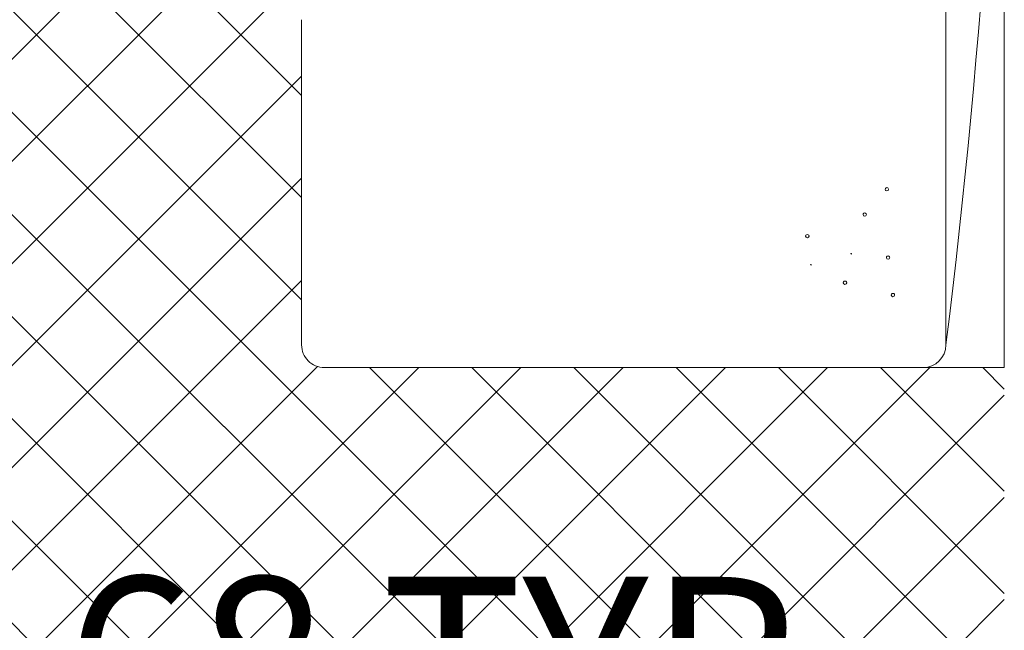
# Model space of a CAD drawing. Units: inches. Extents: x -466983 to 1020, y 324 to 318697.
# Tile 88 of 97: x 776 to 810, y 879 to 900. Entities that reach past the tile are written whole.
import ezdxf

# ---------------------------------------------------------------- set-up
doc = ezdxf.new("R2010")
doc.units = ezdxf.units.IN
doc.header["$MEASUREMENT"] = 0
for name, color, linetype, lineweight in [('A-ANNO-DIMS', 2, 'Continuous', 18), ('A-FLOR-PATT', 252, 'Continuous', 13), ('A-FURN', 8, 'Continuous', 18)]:
    doc.layers.add(name, color=color, linetype=linetype, lineweight=lineweight)
doc.styles.get("Standard").update_dxf_attribs({"font": 'arial.ttf'})
doc.dimstyles.get("Standard").update_dxf_attribs({"dimtxt": 6, "dimasz": 4, "dimexe": 3, "dimexo": 3, "dimgap": 0.09, "dimtad": 0, "dimtih": 1, "dimtoh": 1, "dimdec": 1, "dimzin": 0, "dimdsep": 46, "dimlunit": 3, "dimtxsty": 'Standard', "dimcen": 0.09, "dimadec": 0, "dimazin": 0, "dimtfac": 1, "dimtdec": 1, "dimtofl": 0, "dimtmove": 0, "dimatfit": 3, "dimfxl": 1, "dimtolj": 1, "dimtzin": 0, "dimarcsym": 0})

# ---------------------------------------------------------------- blocks, each defined once
blk = doc.blocks.new('L Shaped Sofa')
at = {"ltscale": 2}
for p, q in [((2356.696, 767.567), (2377.232, 767.567)), ((2355.263, 760.482), (2355.263, 766.134)), ((2355.263, 760.482), (2355.263, 736.259)), ((2355.263, 728.35), (2355.263, 736.259)), ((2355.263, 723.229), (2355.263, 728.35)), ((2356.696, 726.917), (2377.232, 726.917)), ((2393.28, 726.917), (2377.232, 726.917)), ((2355.263, 723.229), (2377.232, 723.229)), ((2475.263, 723.229), (2377.232, 723.229))]:
    blk.add_line(p, q, dxfattribs=at)
for centre, radius, start, end in [((2356.696, 766.134), 1.433, 90, 180), ((2363.564, 735.657), 0.106, 90, 270), ((2363.564, 735.657), 0.106, 270, 90), ((2361.755, 735.431), 0.0177, 90, 270), ((2361.755, 735.431), 0.0177, 270, 90), ((2360.624, 733.281), 0.106, 90, 270), ((2360.624, 733.281), 0.106, 270, 90), ((2362.453, 732.887), 0.0177, 90, 270), ((2362.453, 732.887), 0.0177, 270, 90), ((2364.92, 732.036), 0.106, 90, 270), ((2364.92, 732.036), 0.106, 270, 90), ((2362.207, 730.566), 0.106, 90, 270), ((2362.207, 730.566), 0.106, 270, 90), ((2366.526, 730.64), 0.106, 90, 270), ((2366.526, 730.64), 0.106, 270, 90), ((2359.842, 730.258), 0.106, 90, 270), ((2359.842, 730.258), 0.106, 270, 90), ((2356.696, 728.35), 1.433, 180, 270), ((2416.36, 1205.029), 481.82, 262.88673, 276.63201)]:
    blk.add_arc(centre, radius, start, end, dxfattribs=at)
blk = doc.blocks.new('*D71')
at = {"layer": 'A-ANNO-DIMS', "color": 0, "lineweight": -2, "transparency": 16777216}
for p, q in [((742.215, 885.152), (742.215, 874.91)), ((810.492, 885.152), (810.492, 874.91)), ((738.215, 877.91), (734.215, 877.91)), ((814.492, 877.91), (818.492, 877.91))]:
    blk.add_line(p, q, dxfattribs=at)
at = {"layer": 'A-ANNO-DIMS', "color": 0, "transparency": 16777216}
for points in [[(738.215, 878.577), (738.215, 877.244), (742.215, 877.91)], [(814.492, 878.577), (814.492, 877.244), (810.492, 877.91)]]:
    blk.add_solid(points, dxfattribs=at)
at = {"layer": 'Defpoints', "color": 0, "transparency": 16777216}
for p in [(742.215, 888.152), (810.492, 888.152), (742.215, 877.91)]:
    blk.add_point(p, dxfattribs=at)
at = {"layer": 'A-ANNO-DIMS', "color": 0, "transparency": 16777216, "insert": (776.354, 877.91), "char_height": 6, "attachment_point": 5}
blk.add_mtext('\\A1;L-SOFA 68 TYP.', dxfattribs=at)

msp = doc.modelspace()

# ---------------------------------------------------------------- hatches: boundary and pattern name
at = {"layer": 'A-FLOR-PATT', "transparency": 33554572}
h = msp.add_hatch(dxfattribs=at)
h.set_pattern_fill('ANSI37', color=256, scale=30)
h.set_pattern_definition([(45, (-1212.4137, -290.035), (-2.6516504, 2.6516504), []), (135, (-1212.4137, -290.035), (-2.6516504, -2.6516504), [])])
h.paths.add_polyline_path([(901.806, 1075.938), (900.614, 1075.938), (900.614, 1065.386), (899.391, 1065.386), (898.091, 1065.386), (892.836, 1058.71, -0.258377), (892.188, 1058.351), (879.985, 1058.351, -0.20177), (879.438, 1058.581), (874.081, 1065.386), (872.781, 1065.386), (871.558, 1065.386), (871.558, 1075.938), (813.806, 1075.938), (813.806, 1044.792), (832.395, 1044.792, -0.394795), (848.66, 1028.536), (848.66, 1009.938), (901.806, 1009.938), (901.806, 1015.938), (901.306, 1015.938), (871.306, 1015.938), (871.306, 1017.25), (871.334, 1017.25, -0.401453), (901.306, 1045.938), (901.806, 1045.938)])
edge = h.paths.add_edge_path(flags=16)
edge.add_line((847.773, 1068.949), (847.773, 1073.709))
edge.add_arc((849.227, 1073.709), 1.454, 90, 180, ccw=False)
edge.add_line((849.227, 1075.163), (864.492, 1075.163))
edge.add_arc((864.492, 1073.709), 1.454, 0, 90, ccw=False)
edge.add_line((865.946, 1073.709), (865.946, 1069.004))
edge.add_arc((832.645, 1068.976), 33.301, -20.6123, 0.0472, ccw=False)
edge.add_ellipse((856.859, 1058.48), major_axis=(0, 10.213), ratio=0.685919, start_angle=100.0088, end_angle=259.9912, ccw=False)
edge.add_arc((881.074, 1068.976), 33.301, 180.0472, 200.6123, ccw=False)
h.paths.add_polyline_path([(853.146, 1066.482), (853.146, 1066.453), (853.146, 1066.453, 0.433107), (852.917, 1066.685), (852.917, 1066.453), (853.146, 1066.453), (853.146, 1066.482), (853.088, 1066.612, 0.697939), (852.7, 1066.453), (852.7, 1066.453), (852.7, 1066.482), (852.917, 1067.001), (852.917, 1066.685, -0.396254)], flags=0)
h.paths.add_polyline_path([(861.019, 1066.482), (861.019, 1066.453), (861.019, 1066.453, 0.416404), (860.802, 1066.685), (860.802, 1066.453), (861.019, 1066.453), (861.019, 1066.482), (860.967, 1066.605, 0.713344), (860.573, 1066.453), (860.573, 1066.453), (860.573, 1066.482), (860.802, 1067.001), (860.802, 1066.685, -0.379973)], flags=0)
edge = h.paths.add_edge_path(flags=0)
edge.add_spline(control_points=[(861.13, 1065.785), (861.466, 1065.248), (861.613, 1065.016), (861.983, 1064.374), (862.192, 1063.944), (862.561, 1063.039), (862.721, 1062.563), (862.987, 1061.578), (863.092, 1061.069), (863.245, 1060.031), (863.293, 1059.503), (863.329, 1058.441), (863.318, 1057.908), (863.237, 1056.852), (863.166, 1056.329), (862.97, 1055.308), (862.843, 1054.81), (862.537, 1053.852), (862.357, 1053.393), (861.951, 1052.525), (861.725, 1052.117), (861.233, 1051.362), (860.967, 1051.016), (860.405, 1050.395), (860.108, 1050.12), (859.494, 1049.646), (859.176, 1049.448), (858.528, 1049.13), (858.197, 1049.011), (857.531, 1048.852), (857.196, 1048.812), (856.525, 1048.812), (856.189, 1048.852), (855.524, 1049.01), (855.193, 1049.129), (854.545, 1049.447), (854.227, 1049.645), (853.612, 1050.118), (853.316, 1050.393), (852.753, 1051.014), (852.487, 1051.36), (851.995, 1052.114), (851.769, 1052.523), (851.363, 1053.39), (851.183, 1053.85), (850.877, 1054.807), (850.75, 1055.305), (850.553, 1056.326), (850.483, 1056.849), (850.401, 1057.905), (850.39, 1058.438), (850.426, 1059.5), (850.473, 1060.028), (850.626, 1061.066), (850.732, 1061.575), (850.997, 1062.561), (851.157, 1063.036), (851.525, 1063.942), (851.734, 1064.371), (852.106, 1065.016), (852.254, 1065.25), (852.608, 1065.733)], knot_values=[3.915332, 3.915332, 3.915332, 3.915332, 4.013468, 4.013468, 4.175532, 4.175532, 4.337596, 4.337596, 4.49966, 4.49966, 4.661724, 4.661724, 4.823788, 4.823788, 4.985852, 4.985852, 5.147916, 5.147916, 5.30998, 5.30998, 5.472044, 5.472044, 5.634109, 5.634109, 5.796173, 5.796173, 5.958237, 5.958237, 6.120301, 6.120301, 6.282365, 6.282365, 6.444429, 6.444429, 6.606493, 6.606493, 6.768557, 6.768557, 6.930621, 6.930621, 7.092685, 7.092685, 7.254749, 7.254749, 7.416813, 7.416813, 7.578878, 7.578878, 7.740942, 7.740942, 7.903006, 7.903006, 8.06507, 8.06507, 8.227134, 8.227134, 8.389198, 8.389198, 8.551262, 8.551262, 8.65037, 8.65037, 8.65037, 8.65037], degree=3, periodic=0)
edge.add_line((852.642, 1065.785), (861.13, 1065.785))
edge = h.paths.add_edge_path(flags=0)
edge.add_ellipse((856.85, 1057.743), major_axis=(0, 7.792), ratio=0.687861, start_angle=0, end_angle=360)
h.paths.add_polyline_path([(848.863, 1069.389), (848.863, 1073.96, -0.414214), (849.954, 1075.051), (863.765, 1075.051, -0.414214), (864.856, 1073.96), (864.856, 1069.389, -0.388936), (864.524, 1069.027, -0.043561), (849.195, 1069.027, -0.388936)], flags=0)
h.paths.add_polyline_path([(853.101, 1068.112, -1), (852.677, 1068.112, -1)], flags=0)
edge = h.paths.add_edge_path(flags=0)
edge.add_ellipse((856.859, 1057.338), major_axis=(0, 2.207), ratio=0.657164, start_angle=0, end_angle=360)
h.paths.add_polyline_path([(861.041, 1068.112, -1), (860.618, 1068.112, -1)], flags=0)
edge = h.paths.add_edge_path()
edge.add_line((573.954, 1057.341), (573.954, 1075.938))
edge.add_line((573.954, 1075.938), (558.731, 1075.938))
edge.add_line((558.731, 1075.938), (558.731, 1065.386))
edge.add_line((558.731, 1065.386), (557.507, 1065.386))
edge.add_line((557.507, 1065.386), (556.207, 1065.386))
edge.add_line((556.207, 1065.386), (550.952, 1058.71))
edge.add_arc((550.304, 1059.116), 0.765, 270, 327.9483, ccw=False)
edge.add_line((550.304, 1058.351), (538.101, 1058.351))
edge.add_arc((538.101, 1059.116), 0.765, 224.3704, 270, ccw=False)
edge.add_line((537.555, 1058.581), (532.198, 1065.386))
edge.add_line((532.198, 1065.386), (530.898, 1065.386))
edge.add_line((530.898, 1065.386), (529.674, 1065.386))
edge.add_line((529.674, 1065.386), (529.674, 1075.938))
edge.add_line((529.674, 1075.938), (520.806, 1075.938))
edge.add_line((520.806, 1075.938), (520.806, 1045.938))
edge.add_line((520.806, 1045.938), (521.306, 1045.938))
edge.add_arc((521.306, 1015.938), 30, 2.5075, 90, ccw=False)
edge.add_line((551.277, 1017.25), (551.306, 1017.25))
edge.add_line((551.306, 1017.25), (551.306, 1015.938))
edge.add_line((551.306, 1015.938), (520.806, 1015.938))
edge.add_line((520.806, 1015.938), (520.806, 1009.938))
edge.add_line((520.806, 1009.938), (559.191, 1010.402))
edge.add_arc((559.191, 1011.856), 1.454, 180, 270, ccw=False)
edge.add_line((557.737, 1011.856), (557.737, 1016.561))
edge.add_arc((591.039, 1016.589), 33.301, 159.3877, 180.0472, ccw=False)
edge.add_ellipse((566.824, 1027.085), major_axis=(0, 10.213), ratio=0.685919, start_angle=280.0088, end_angle=439.9912, ccw=False)
edge.add_arc((542.609, 1016.589), 33.301, 0.0472, 20.6123, ccw=False)
edge.add_line((575.91, 1016.616), (575.91, 1011.856))
edge.add_arc((574.456, 1011.856), 1.454, -90, 0, ccw=False)
edge.add_line((574.456, 1010.402), (608.806, 1009.938))
edge.add_line((608.806, 1009.938), (608.806, 1041.086))
edge.add_line((608.806, 1041.086), (590.218, 1041.086))
edge.add_arc((590.775, 1057.907), 16.831, 181.9277, 268.1032, ccw=False)
edge = h.paths.add_edge_path()
edge.add_ellipse((494.244, 583.62), major_axis=(0, 10.213), ratio=0.685919, start_angle=280.0088, end_angle=439.9912, ccw=False)
edge.add_arc((470.03, 573.124), 33.301, 0.0472, 20.6123, ccw=False)
edge.add_line((503.331, 573.152), (503.331, 568.392))
edge.add_arc((501.877, 568.392), 1.454, -90, 0, ccw=False)
edge.add_line((501.877, 566.938), (539.806, 566.938))
edge.add_line((539.806, 566.938), (539.806, 572.938))
edge.add_line((539.806, 572.938), (539.306, 572.938))
edge.add_line((539.306, 572.938), (509.306, 572.938))
edge.add_line((509.306, 572.938), (509.306, 574.25))
edge.add_line((509.306, 574.25), (509.334, 574.25))
edge.add_arc((539.306, 572.938), 30, 90, 177.4925, ccw=False)
edge.add_line((539.306, 602.938), (539.806, 602.938))
edge.add_line((539.806, 602.938), (539.806, 626.938))
edge.add_line((539.806, 626.938), (531.772, 626.938))
edge.add_line((531.772, 626.938), (531.772, 616.386))
edge.add_line((531.772, 616.386), (530.548, 616.386))
edge.add_line((530.548, 616.386), (529.249, 616.386))
edge.add_line((529.249, 616.386), (523.711, 609.351))
edge.add_line((523.711, 609.351), (510.777, 609.351))
edge.add_line((510.777, 609.351), (505.239, 616.386))
edge.add_line((505.239, 616.386), (503.939, 616.386))
edge.add_line((503.939, 616.386), (502.715, 616.386))
edge.add_line((502.715, 616.386), (502.715, 626.938))
edge.add_line((502.715, 626.938), (481.698, 626.938))
edge.add_line((481.698, 626.938), (481.698, 610.995))
edge.add_arc((467.27, 611.473), 14.436, 271.9277, 358.1032, ccw=False)
edge.add_line((467.756, 597.045), (451.806, 597.045))
edge.add_line((451.806, 597.045), (451.806, 584.404))
edge.add_line((451.806, 584.404), (451.806, 566.938))
edge.add_line((451.806, 566.938), (486.612, 566.938))
edge.add_arc((486.612, 568.392), 1.454, 180, 270, ccw=False)
edge.add_line((485.158, 568.392), (485.158, 573.097))
edge.add_arc((518.459, 573.124), 33.301, 159.3877, 180.0472, ccw=False)
h.paths.add_polyline_path([(836.261, 1020.733), (879.89, 1020.733), (879.89, 1039.39), (836.261, 1039.39)], flags=25)
h.paths.add_polyline_path([(549.985, 1036.749), (593.614, 1036.749), (593.614, 1055.407), (549.985, 1055.407)], flags=24)
h.paths.add_polyline_path([(475.123, 595.596), (518.752, 595.596), (518.752, 614.253), (475.123, 614.253)], flags=24)
h = msp.add_hatch(dxfattribs=at)
h.set_pattern_fill('ANSI37', color=256, scale=20)
h.set_pattern_definition([(45, (-1212.4137, -290.035), (-1.767767, 1.767767), []), (135, (-1212.4137, -290.035), (-1.767767, -1.767767), [])])
h.paths.add_polyline_path([(809.806, 870.938), (809.806, 888.152), (806.998, 888.152), (802.662, 888.152), (789.383, 888.152), (786.285, 888.152, -0.414214), (785.499, 888.937), (785.499, 900.196), (785.499, 908.47, -0.414214), (786.808, 909.779, -0.414214), (785.499, 911.088), (785.499, 929.101, -0.414214), (786.808, 930.411, -0.414214), (785.499, 931.72), (785.499, 931.904, -0.414214), (784.19, 930.595), (766.722, 930.595, -0.412359), (765.413, 931.896, -0.413741), (764.115, 930.578), (744.578, 930.422, -0.416556), (743.786, 931.207), (743.786, 933.515), (742.215, 933.515), (742.215, 952.024, -0.001344), (743.786, 952.2), (743.786, 953.938), (678.592, 953.938), (678.592, 951.131), (678.592, 946.794), (678.592, 933.515), (678.592, 930.417, -0.414214), (677.806, 929.631), (666.548, 929.631), (658.274, 929.631, -0.414214), (656.965, 930.94, -0.414214), (655.656, 929.631), (637.642, 929.631, -0.414214), (636.333, 930.94, -0.414214), (635.024, 929.631), (634.839, 929.631, -0.414214), (636.149, 928.322), (636.149, 910.854, -0.412359), (634.848, 909.545, -0.413741), (636.165, 908.247), (636.321, 888.71, -0.416556), (635.536, 887.918), (633.228, 887.918), (633.228, 886.347), (614.719, 886.347, -0.001344), (614.544, 887.918), (612.806, 887.918), (612.806, 834.938), (612.806, 752.938), (612.806, 748.938), (612.806, 697.938), (654.806, 697.938), (654.806, 701.938), (715.806, 701.938), (715.806, 737.435), (774.292, 737.435), (774.292, 795.938), (809.806, 795.938)])
h.paths.add_polyline_path([(679.276, 849.576, 0.102523), (682.148, 849.261, -0.080461), (694.543, 849.773, -0.283899), (694.482, 849.008, 0.136605), (694.407, 848.81, -0.030441), (694.543, 846.893), (694.543, 842.62), (694.543, 838.347, -0.028219), (694.425, 836.568), (694.425, 836.568, 0.196187), (694.446, 836.271, -0.302897), (694.543, 835.467, -0.080461), (682.148, 835.979, 0.102523), (679.276, 835.664, -0.58611), (678.646, 836.017), (678.646, 849.223, -0.58611)], flags=16)
h.paths.add_polyline_path([(679.517, 848.651, 0.699597), (679.476, 848.634, 1.20716), (679.194, 848.742, 0.010621)], flags=0)
h.paths.add_polyline_path([(679.492, 836.561, -0.013798), (679.918, 836.659, -0.071703), (682.853, 837.143, -0.165743), (682.166, 839.101), (682.166, 842.609), (682.166, 846.06, -0.240616), (683.473, 848.677, -0.068263), (693.929, 849.008), (693.788, 848.708), (693.788, 849.023, 0.067332), (683.473, 848.677, 0.240616), (682.166, 846.06), (682.166, 842.609), (682.166, 839.101, 0.23459), (683.461, 836.551, 0.068093), (693.788, 836.195), (693.788, 836.51), (693.93, 836.21, -0.077215), (682.242, 836.782, 0.086627), (679.528, 836.57, -0.628402), (679.503, 836.573), (679.503, 836.607, 0.910458)], flags=0)
h.paths.add_polyline_path([(679.476, 848.636), (679.207, 848.647), (679.207, 836.572, 0.913566), (679.365, 836.586), (679.476, 836.582)], flags=0)
h.paths.add_polyline_path([(679.276, 829.86, 0.102523), (682.148, 829.546, -0.080461), (694.543, 830.057, -0.283899), (694.482, 829.293, 0.136605), (694.407, 829.095, -0.030441), (694.543, 827.178), (694.543, 822.904), (694.543, 818.631, -0.028219), (694.425, 816.853), (694.425, 816.853, 0.196187), (694.446, 816.556, -0.302897), (694.543, 815.752, -0.080461), (682.148, 816.263, 0.102523), (679.276, 815.949, -0.58611), (678.646, 816.302), (678.646, 829.507, -0.58611)], flags=16)
h.paths.add_polyline_path([(679.517, 828.936, 0.699597), (679.476, 828.919, 1.20716), (679.194, 829.027, 0.010621)], flags=0)
h.paths.add_polyline_path([(679.492, 816.846, -0.013798), (679.918, 816.944, -0.071703), (682.853, 817.428, -0.165743), (682.166, 819.385), (682.166, 822.894), (682.166, 826.345, -0.240616), (683.473, 828.961, -0.068263), (693.929, 829.293), (693.788, 828.993), (693.788, 829.308, 0.067332), (683.473, 828.961, 0.240616), (682.166, 826.345), (682.166, 822.894), (682.166, 819.385, 0.23459), (683.461, 816.836, 0.068093), (693.788, 816.48), (693.788, 816.795), (693.93, 816.495, -0.077215), (682.242, 817.066, 0.086627), (679.528, 816.855, -0.628402), (679.503, 816.858), (679.503, 816.892, 0.910458)], flags=0)
h.paths.add_polyline_path([(679.476, 828.921), (679.207, 828.932), (679.207, 816.857, 0.913566), (679.365, 816.871), (679.476, 816.867)], flags=0)
h.paths.add_polyline_path([(679.276, 810.145, 0.102523), (682.148, 809.83, -0.080461), (694.543, 810.342, -0.3023), (694.447, 809.539, 0.10023), (694.406, 809.388, -0.03057), (694.543, 807.462), (694.543, 803.189), (694.543, 798.916, -0.03057), (694.406, 796.991, 0.10023), (694.447, 796.839, -0.3023), (694.543, 796.036, -0.080461), (682.148, 796.548, 0.102523), (679.276, 796.233, -0.58611), (678.646, 796.586), (678.646, 809.792, -0.58611)], flags=16)
h.paths.add_polyline_path([(679.517, 809.242, 0.699597), (679.476, 809.224, 1.20716), (679.194, 809.332, 0.010621)], flags=0)
h.paths.add_polyline_path([(679.492, 797.151, -0.013798), (679.918, 797.25, -0.071703), (682.853, 797.734, -0.165743), (682.166, 799.691), (682.166, 803.2), (682.166, 806.65, -0.239349), (683.461, 809.258, -0.072465), (694.447, 809.541, 0.197932), (694.425, 809.241), (693.788, 809.299), (693.788, 809.614, 0.068093), (683.461, 809.258, 0.239349), (682.166, 806.65), (682.166, 803.2), (682.166, 799.691, 0.235854), (683.473, 797.132, 0.067332), (693.788, 796.786), (693.788, 797.101), (694.425, 797.159, 0.197932), (694.447, 796.859, -0.080419), (682.156, 797.379, 0.083867), (679.528, 797.16, -0.628402), (679.503, 797.164), (679.503, 797.197, 0.910458)], flags=0)
h.paths.add_polyline_path([(679.207, 809.237), (679.207, 797.162, 0.913566), (679.365, 797.176), (679.476, 797.173), (679.476, 809.227)], flags=0)
h.paths.add_polyline_path([(695.364, 853.299), (728.223, 853.299), (728.223, 771.152), (695.364, 771.152)], flags=16)
h.paths.add_polyline_path([(696.021, 852.642), (727.566, 852.642), (727.566, 771.809), (696.021, 771.809)], flags=0)
h.paths.add_polyline_path([(679.276, 788.787, 0.102523), (682.148, 788.472, -0.080461), (694.543, 788.984, -0.3023), (694.447, 788.181, 0.10023), (694.406, 788.03, -0.03057), (694.543, 786.104), (694.543, 781.831), (694.543, 777.558, -0.03057), (694.406, 775.632, 0.10023), (694.447, 775.481, -0.3023), (694.543, 774.678, -0.080461), (682.148, 775.19, 0.102523), (679.276, 774.875, -0.58611), (678.646, 775.228), (678.646, 788.434, -0.58611)], flags=16)
h.paths.add_polyline_path([(679.517, 787.883, 0.699597), (679.476, 787.866, 1.20716), (679.194, 787.974, 0.010621)], flags=0)
h.paths.add_polyline_path([(679.492, 775.793, -0.013798), (679.918, 775.891, -0.071703), (682.853, 776.375, -0.165743), (682.166, 778.333), (682.166, 781.841), (682.166, 785.292, -0.239349), (683.461, 787.899, -0.072465), (694.447, 788.182, 0.197932), (694.425, 787.882), (693.788, 787.94), (693.788, 788.255, 0.068093), (683.461, 787.899, 0.239349), (682.166, 785.292), (682.166, 781.841), (682.166, 778.333, 0.235854), (683.473, 775.774, 0.067332), (693.788, 775.428), (693.788, 775.742), (694.425, 775.8, 0.197932), (694.447, 775.5, -0.080419), (682.156, 776.021, 0.083867), (679.528, 775.802, -0.628402), (679.503, 775.805), (679.503, 775.839, 0.910458)], flags=0)
h.paths.add_polyline_path([(679.207, 787.879), (679.207, 775.804, 0.913566), (679.365, 775.818), (679.476, 775.814), (679.476, 787.868)], flags=0)
h.paths.add_polyline_path([(704.641, 854.12, -0.080461), (705.153, 866.516, 0.102523), (704.838, 869.387, -0.58611), (705.191, 870.017), (718.397, 870.017, -0.58611), (718.75, 869.387, 0.102523), (718.435, 866.516, -0.080461), (718.946, 854.12, -0.3023), (718.144, 854.217, 0.10023), (717.992, 854.257, -0.03057), (716.067, 854.12), (711.794, 854.12), (707.521, 854.12, -0.03057), (705.595, 854.257, 0.10023), (705.444, 854.217, -0.3023)], flags=16)
h.paths.add_polyline_path([(717.846, 869.146, 0.699597), (717.829, 869.187, 1.20716), (717.937, 869.47, 0.010621)], flags=0)
h.paths.add_polyline_path([(705.463, 854.216, -0.080419), (705.984, 866.507, 0.083867), (705.765, 869.135, -0.628402), (705.768, 869.16), (705.802, 869.16, 0.910458), (705.756, 869.171, -0.013798), (705.854, 868.745, -0.071703), (706.338, 865.81, -0.165743), (708.295, 866.497), (711.804, 866.497), (715.255, 866.497, -0.239349), (717.862, 865.202, -0.072465), (718.145, 854.216, 0.197932), (717.845, 854.238), (717.903, 854.876), (718.218, 854.876, 0.068093), (717.862, 865.202, 0.239349), (715.255, 866.497), (711.804, 866.497), (708.295, 866.497, 0.235854), (705.737, 865.19, 0.067332), (705.391, 854.876), (705.705, 854.876), (705.763, 854.238, 0.197932)], flags=16)
h.paths.add_polyline_path([(705.766, 869.456, 0.913566), (705.781, 869.299), (705.777, 869.187), (717.831, 869.187), (717.842, 869.456)], flags=0)
h.paths.add_polyline_path([(729.045, 842.62), (729.045, 846.893, -0.03057), (729.182, 848.818, 0.10023), (729.141, 848.97, -0.3023), (729.045, 849.773, -0.080461), (741.44, 849.261, 0.102523), (744.311, 849.576, -0.58611), (744.942, 849.223), (744.942, 836.017, -0.58611), (744.311, 835.664, 0.102523), (741.44, 835.979, -0.080461), (729.045, 835.467, -0.3023), (729.141, 836.27, 0.10023), (729.182, 836.421, -0.03057), (729.045, 838.347)], flags=16)
h.paths.add_polyline_path([(744.111, 836.585, 1.20716), (744.394, 836.477, 0.010621), (744.07, 836.567, 0.699597)], flags=0)
h.paths.add_polyline_path([(729.141, 836.268, 0.197932), (729.162, 836.568), (729.8, 836.51), (729.8, 836.195, 0.068093), (740.126, 836.551, 0.239349), (741.421, 839.159), (741.421, 842.609), (741.421, 846.118, 0.235854), (740.114, 848.677, 0.067332), (729.8, 849.023), (729.8, 848.708), (729.162, 848.65, 0.197932), (729.141, 848.95, -0.080419), (741.432, 848.43, 0.083867), (744.059, 848.649, -0.628402), (744.085, 848.645), (744.085, 848.612, 0.910458), (744.095, 848.658, -0.013798), (743.67, 848.559, -0.071703), (740.734, 848.075, -0.165743), (741.421, 846.118), (741.421, 842.609), (741.421, 839.159, -0.239349), (740.126, 836.551, -0.072465)], flags=0)
h.paths.add_polyline_path([(729.045, 830.057, -0.080461), (741.44, 829.546, 0.102523), (744.311, 829.86, -0.58611), (744.942, 829.507), (744.942, 816.302, -0.58611), (744.311, 815.949, 0.102523), (741.44, 816.263, -0.080461), (729.045, 815.752, -0.3023), (729.141, 816.554, 0.10023), (729.182, 816.706, -0.03057), (729.045, 818.631), (729.045, 822.904), (729.045, 827.178, -0.03057), (729.182, 829.103, 0.10023), (729.141, 829.255, -0.3023)], flags=16)
h.paths.add_polyline_path([(744.111, 816.869, 1.20716), (744.394, 816.761, 0.010621), (744.07, 816.852, 0.699597)], flags=0)
h.paths.add_polyline_path([(729.141, 829.235, -0.080419), (741.432, 828.714, 0.083867), (744.059, 828.933, -0.628402), (744.085, 828.93), (744.085, 828.896, 0.910458), (744.095, 828.943, -0.013798), (743.67, 828.844, -0.071703), (740.734, 828.36, -0.165743), (741.421, 826.403), (741.421, 822.894), (741.421, 819.443, -0.239349), (740.126, 816.836, -0.072465), (729.141, 816.553, 0.197932), (729.162, 816.853), (729.8, 816.795), (729.8, 816.48, 0.068093), (740.126, 816.836, 0.239349), (741.421, 819.443), (741.421, 822.894), (741.421, 826.403, 0.235854), (740.114, 828.961, 0.067332), (729.8, 829.308), (729.8, 828.993), (729.162, 828.935, 0.197932)], flags=16)
h.paths.add_polyline_path([(729.045, 810.342, -0.080461), (741.44, 809.83, 0.102523), (744.311, 810.145, -0.58611), (744.942, 809.792), (744.942, 796.586, -0.58611), (744.311, 796.233, 0.102523), (741.44, 796.548, -0.080461), (729.045, 796.036, -0.283899), (729.105, 796.801, 0.136605), (729.181, 796.999, -0.030441), (729.045, 798.916), (729.045, 803.189), (729.045, 807.462, -0.028219), (729.163, 809.241), (729.162, 809.241, 0.196187), (729.142, 809.538, -0.302897)], flags=16)
h.paths.add_polyline_path([(744.111, 797.175, 1.20716), (744.394, 797.067, 0.010621), (744.07, 797.158, 0.699597)], flags=0)
h.paths.add_polyline_path([(741.345, 809.027, 0.086627), (744.059, 809.239, -0.628402), (744.085, 809.235), (744.085, 809.202, 0.910458), (744.095, 809.248, -0.013798), (743.67, 809.15, -0.071703), (740.734, 808.666, -0.165743), (741.421, 806.708), (741.421, 803.2), (741.421, 799.749, -0.240616), (740.114, 797.132, -0.068263), (729.658, 796.801), (729.8, 797.101), (729.8, 796.786, 0.067332), (740.114, 797.132, 0.240616), (741.421, 799.749), (741.421, 803.2), (741.421, 806.708, 0.23459), (740.126, 809.258, 0.068093), (729.8, 809.614), (729.8, 809.299), (729.658, 809.599, -0.077215)], flags=0)
h.paths.add_polyline_path([(704.641, 770.33, -0.283899), (705.405, 770.27, 0.136605), (705.603, 770.194, -0.030441), (707.521, 770.33), (711.794, 770.33), (716.067, 770.33, -0.028219), (717.845, 770.212), (717.845, 770.213, 0.196187), (718.143, 770.233, -0.302897), (718.946, 770.33, -0.080461), (718.435, 757.935, 0.102523), (718.75, 755.064, -0.58611), (718.397, 754.433), (705.191, 754.433, -0.58611), (704.838, 755.064, 0.102523), (705.153, 757.935, -0.080461)], flags=16)
h.paths.add_polyline_path([(705.762, 755.305, 0.699597), (705.779, 755.264, 1.20716), (705.671, 754.981, 0.010621)], flags=0)
h.paths.add_polyline_path([(705.405, 769.717), (705.705, 769.575), (705.391, 769.575, 0.067332), (705.737, 759.261, 0.240616), (708.353, 757.954), (711.804, 757.954), (715.313, 757.954, 0.23459), (717.862, 759.249, 0.068093), (718.218, 769.575), (717.903, 769.575), (718.203, 769.717, -0.077215), (717.632, 758.03, 0.086627), (717.843, 755.316, -0.628402), (717.84, 755.29), (717.806, 755.29, 0.910458), (717.853, 755.28, -0.013798), (717.754, 755.705, -0.071703), (717.27, 758.641, -0.165743), (715.313, 757.954), (711.804, 757.954), (708.353, 757.954, -0.240616), (705.737, 759.261, -0.068263)], flags=0)
h.paths.add_polyline_path([(729.045, 788.984, -0.080461), (741.44, 788.472, 0.102523), (744.311, 788.787, -0.58611), (744.942, 788.434), (744.942, 775.228, -0.58611), (744.311, 774.875, 0.102523), (741.44, 775.19, -0.080461), (729.045, 774.678, -0.283899), (729.105, 775.443, 0.136605), (729.181, 775.64, -0.030441), (729.045, 777.558), (729.045, 781.831), (729.045, 786.104, -0.028219), (729.163, 787.882), (729.162, 787.882, 0.196187), (729.142, 788.18, -0.302897)], flags=16)
h.paths.add_polyline_path([(744.111, 775.817, 1.20716), (744.394, 775.709, 0.010621), (744.07, 775.799, 0.699597)], flags=0)
h.paths.add_polyline_path([(741.345, 787.669, 0.086627), (744.059, 787.881, -0.628402), (744.085, 787.877), (744.085, 787.844, 0.910458), (744.095, 787.89, -0.013798), (743.67, 787.791, -0.071703), (740.734, 787.307, -0.165743), (741.421, 785.35), (741.421, 781.841), (741.421, 778.39, -0.240616), (740.114, 775.774, -0.068263), (729.658, 775.443), (729.8, 775.742), (729.8, 775.428, 0.067332), (740.114, 775.774, 0.240616), (741.421, 778.39), (741.421, 781.841), (741.421, 785.35, 0.23459), (740.126, 787.899, 0.068093), (729.8, 788.255), (729.8, 787.94), (729.658, 788.241, -0.077215)], flags=0)
h.paths.add_polyline_path([(744.111, 848.636), (744.111, 836.582), (744.381, 836.572), (744.381, 848.647, 0.913566), (744.223, 848.633)], flags=0)
h.paths.add_polyline_path([(744.223, 828.917), (744.111, 828.921), (744.111, 816.867), (744.381, 816.857), (744.381, 828.932, 0.913566)], flags=0)
h.paths.add_polyline_path([(717.831, 755.264), (705.777, 755.264), (705.766, 754.994), (717.842, 754.994, 0.913566), (717.827, 755.152)], flags=0)
h.paths.add_polyline_path([(744.223, 809.223), (744.111, 809.227), (744.111, 797.173), (744.381, 797.162), (744.381, 809.237, 0.913566)], flags=0)
h.paths.add_polyline_path([(744.111, 787.868), (744.111, 775.814), (744.381, 775.804), (744.381, 787.879, 0.913566), (744.223, 787.865)], flags=0)
h.paths.add_polyline_path([(678.877, 877.123), (737.613, 877.123), (737.613, 899.512), (678.877, 899.512)], flags=24)

# ---------------------------------------------------------------- block references
at = {"layer": 'A-FURN', "xscale": 0.5482153745360612, "yscale": 0.5482153745360612, "zscale": 0.5482153745360612, "rotation": 89.99999999999999}
msp.add_blockref('L Shaped Sofa', (1206.291, -403.039), dxfattribs=at)

# ---------------------------------------------------------------- dimensions: what is measured, and where the dimension line sits
at = {"layer": 'A-ANNO-DIMS'}
dim = msp.add_linear_dim(base=(742.215, 877.91), p1=(810.492, 888.152), p2=(742.215, 888.152), angle=180, text='L-SOFA <> TYP.', dimstyle='Standard', override={"dimdec": 0, "dimlfac": 1, "dimrnd": 0, "dimzin": 0, "dimdsep": 46, "dimlunit": 2}, dxfattribs=at)
dim.commit()
dim.dimension.update_dxf_attribs({"geometry": '*D71', "text_midpoint": (776.354, 877.91)})

doc.saveas('drawing.dxf')
